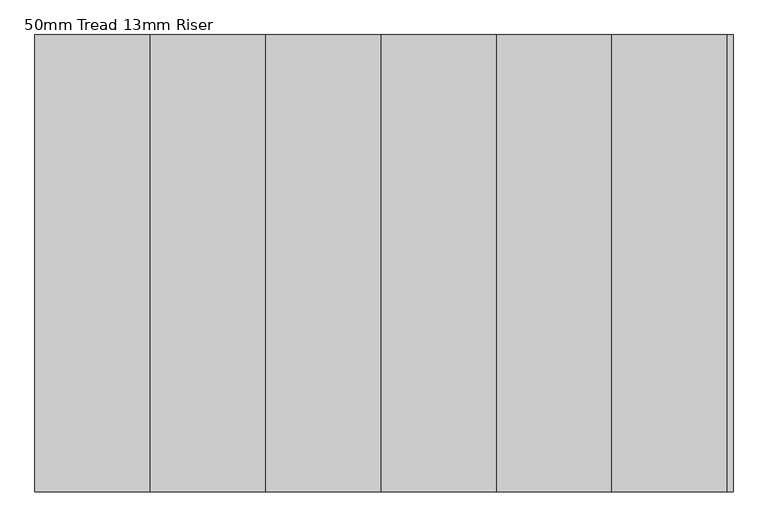
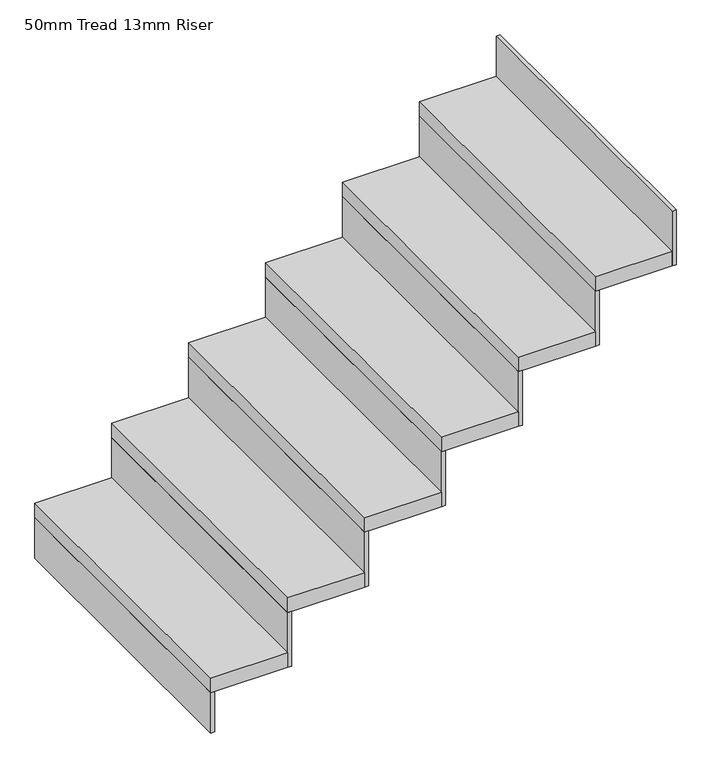
"""IFC4 building model written with IfcOpenShell, lengths in millimetres: stair flight geometry, 50mm Tread 13mm Riser."""

from ifc_helpers import new_model, si_unit, frame, origin, origin_with_axes, place, context, project, spatial, polyline, outline, extrude, source, transform, mapped, element, save


def stair_flight_50mm_tread_13mm_riser_519f3169(model_context):
    return source(origin(), model_context, "Body", "SweptSolid", [
        extrude(outline(polyline([(-11979.6794909, -2498.5618509), (-11992.1794909, -2498.5618509), (-11992.1794909, -1507.9618509), (-11979.6794909, -1507.9618509), (-11979.6794909, -2498.5618509)])), origin_with_axes(), (0.0, 0.0, 1.0), 138.2588235),
        extrude(outline(polyline([(-11742.1794909, -1507.9618509), (-11742.1794909, -2498.5618509), (-11992.1794909, -2498.5618509), (-11992.1794909, -1507.9618509), (-11742.1794909, -1507.9618509)])), frame((0.0, 0.0, 138.2588235), z_axis=(0.0, 0.0, 1.0), x_axis=(1.0, 0.0, 0.0)), (0.0, 0.0, 1.0), 50.0),
        extrude(outline(polyline([(-11729.6794909, -2498.5618509), (-11742.1794909, -2498.5618509), (-11742.1794909, -1507.9618509), (-11729.6794909, -1507.9618509), (-11729.6794909, -2498.5618509)])), frame((0.0, 0.0, 138.2588235), z_axis=(0.0, 0.0, 1.0), x_axis=(1.0, 0.0, 0.0)), (0.0, 0.0, 1.0), 188.2588235),
        extrude(outline(polyline([(-11492.1794909, -1507.9618509), (-11492.1794909, -2498.5618509), (-11742.1794909, -2498.5618509), (-11742.1794909, -1507.9618509), (-11492.1794909, -1507.9618509)])), frame((0.0, 0.0, 326.5176471), z_axis=(0.0, 0.0, 1.0), x_axis=(1.0, 0.0, 0.0)), (0.0, 0.0, 1.0), 50.0),
        extrude(outline(polyline([(-11479.6794909, -2498.5618509), (-11492.1794909, -2498.5618509), (-11492.1794909, -1507.9618509), (-11479.6794909, -1507.9618509), (-11479.6794909, -2498.5618509)])), frame((0.0, 0.0, 326.5176471), z_axis=(0.0, 0.0, 1.0), x_axis=(1.0, 0.0, 0.0)), (0.0, 0.0, 1.0), 188.2588235),
        extrude(outline(polyline([(-11242.1794909, -1507.9618509), (-11242.1794909, -2498.5618509), (-11492.1794909, -2498.5618509), (-11492.1794909, -1507.9618509), (-11242.1794909, -1507.9618509)])), frame((0.0, 0.0, 514.7764706), z_axis=(0.0, 0.0, 1.0), x_axis=(1.0, 0.0, 0.0)), (0.0, 0.0, 1.0), 50.0),
        extrude(outline(polyline([(-11229.6794909, -2498.5618509), (-11242.1794909, -2498.5618509), (-11242.1794909, -1507.9618509), (-11229.6794909, -1507.9618509), (-11229.6794909, -2498.5618509)])), frame((0.0, 0.0, 514.7764706), z_axis=(0.0, 0.0, 1.0), x_axis=(1.0, 0.0, 0.0)), (0.0, 0.0, 1.0), 188.2588235),
        extrude(outline(polyline([(-10992.1794909, -1507.9618509), (-10992.1794909, -2498.5618509), (-11242.1794909, -2498.5618509), (-11242.1794909, -1507.9618509), (-10992.1794909, -1507.9618509)])), frame((0.0, 0.0, 703.0352941), z_axis=(0.0, 0.0, 1.0), x_axis=(1.0, 0.0, 0.0)), (0.0, 0.0, 1.0), 50.0),
        extrude(outline(polyline([(-10979.6794909, -2498.5618509), (-10992.1794909, -2498.5618509), (-10992.1794909, -1507.9618509), (-10979.6794909, -1507.9618509), (-10979.6794909, -2498.5618509)])), frame((0.0, 0.0, 703.0352941), z_axis=(0.0, 0.0, 1.0), x_axis=(1.0, 0.0, 0.0)), (0.0, 0.0, 1.0), 188.2588235),
        extrude(outline(polyline([(-10742.1794909, -1507.9618509), (-10742.1794909, -2498.5618509), (-10992.1794909, -2498.5618509), (-10992.1794909, -1507.9618509), (-10742.1794909, -1507.9618509)])), frame((0.0, 0.0, 891.2941176), z_axis=(0.0, 0.0, 1.0), x_axis=(1.0, 0.0, 0.0)), (0.0, 0.0, 1.0), 50.0),
        extrude(outline(polyline([(-10729.6794909, -2498.5618509), (-10742.1794909, -2498.5618509), (-10742.1794909, -1507.9618509), (-10729.6794909, -1507.9618509), (-10729.6794909, -2498.5618509)])), frame((0.0, 0.0, 891.2941176), z_axis=(0.0, 0.0, 1.0), x_axis=(1.0, 0.0, 0.0)), (0.0, 0.0, 1.0), 188.2588235),
        extrude(outline(polyline([(-10479.6794909, -2498.5618509), (-10492.1794909, -2498.5618509), (-10492.1794909, -1507.9618509), (-10479.6794909, -1507.9618509), (-10479.6794909, -2498.5618509)])), frame((0.0, 0.0, 1079.5529412), z_axis=(0.0, 0.0, 1.0), x_axis=(1.0, 0.0, 0.0)), (0.0, 0.0, 1.0), 188.2588235),
        extrude(outline(polyline([(-10492.1794909, -1507.9618509), (-10492.1794909, -2498.5618509), (-10742.1794909, -2498.5618509), (-10742.1794909, -1507.9618509), (-10492.1794909, -1507.9618509)])), frame((0.0, 0.0, 1079.5529412), z_axis=(0.0, 0.0, 1.0), x_axis=(1.0, 0.0, 0.0)), (0.0, 0.0, 1.0), 50.0),
    ])


if __name__ == "__main__":
    model = new_model("IFC4")
    model_context = context("Model", 3, world=origin())
    ifc_project = project(units=[si_unit("LENGTHUNIT", "METRE", prefix="MILLI")], contexts=[model_context])
    site = spatial("IfcSite", under=ifc_project)
    building = spatial("IfcBuilding", under=site)
    placement = place(None, origin())
    stair_flight_50mm_tread_13mm_riser_shape = stair_flight_50mm_tread_13mm_riser_519f3169(model_context)
    element("IfcStairFlight", 1, ObjectType="50mm Tread 13mm Riser", at=placement, inside=building, context=model_context, shape_type="MappedRepresentation", body=[
        mapped(stair_flight_50mm_tread_13mm_riser_shape, transform((0.0, 0.0, 0.0), x_axis=(1.0, 0.0, 0.0), y_axis=(0.0, 1.0, 0.0), z_axis=(0.0, 0.0, 1.0))),
    ])
    save(model, "model.ifc")
